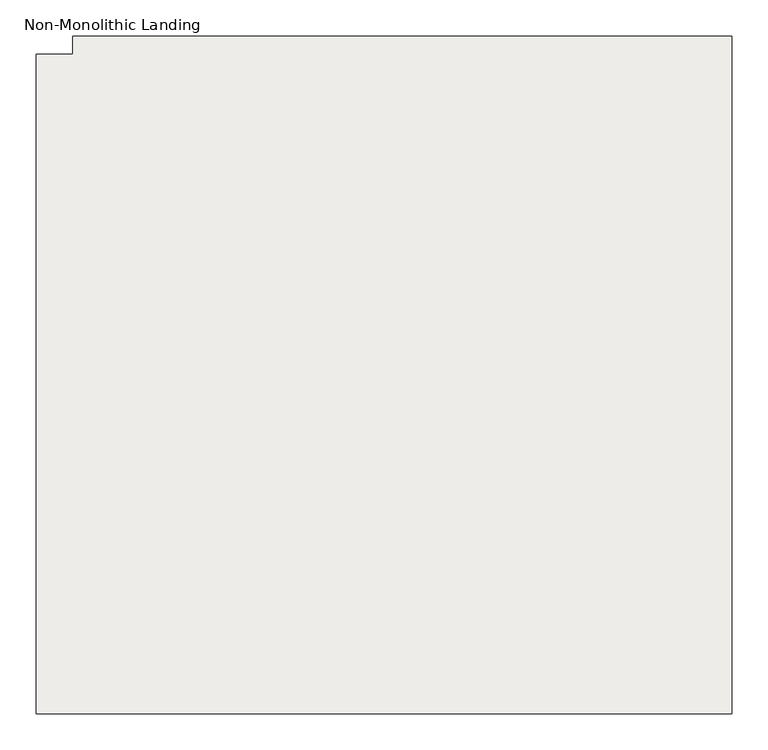
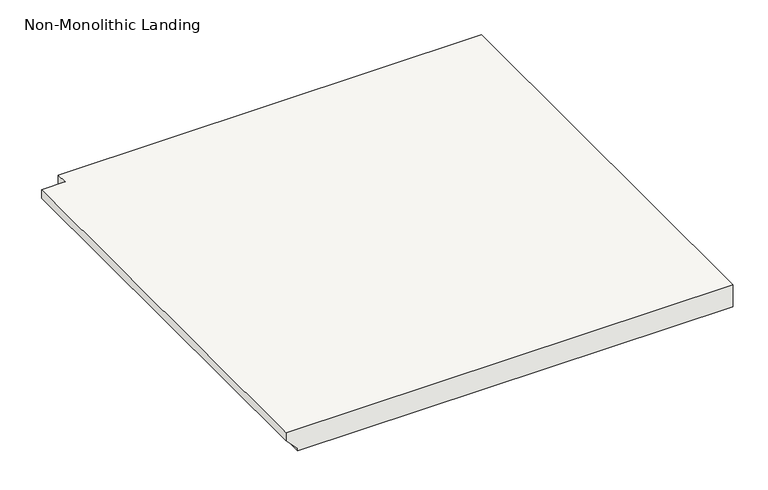
"""IFC4 building model written with IfcOpenShell, lengths in millimetres: slab geometry, Non-Monolithic Landing."""

from ifc_helpers import new_model, si_unit, origin, place, context, project, spatial, faceted_brep, source, transform, mapped, element, save


def non_monolithic_landing_5acc3baf(model_context):
    return source(origin(), model_context, "Body", "Brep", [
        faceted_brep([(-1954.0563134, -12709.459218, 4044.95), (-1954.0563134, -12709.459218, 4064.0), (-1954.0563134, -11795.059218, 4064.0), (-1954.0563134, -11795.059218, 4044.95), (-1928.6563134, -12709.459218, 4019.55), (-1928.6563134, -11795.059218, 4019.55), (-988.8563134, -12709.459218, 4064.0), (-988.8563134, -11795.059218, 4064.0), (-988.8563134, -11769.659218, 4064.0), (-1903.2563134, -11769.659218, 4064.0), (-1903.2563134, -11795.059218, 4064.0), (-1928.6563134, -12709.459218, 4013.2), (-1928.6563134, -11795.059218, 4013.2), (-1903.2563134, -11795.059218, 4013.2), (-1903.2563134, -11769.659218, 4013.2), (-988.8563134, -11769.659218, 4013.2), (-988.8563134, -11795.059218, 4013.2), (-988.8563134, -12709.459218, 4013.2)], [[[0, 1, 2, 3]], [[4, 0, 3, 5]], [[6, 7, 8, 9, 10, 2, 1]], [[11, 12, 13, 14, 15, 16, 17]], [[12, 11, 4, 5]], [[6, 1, 0, 4, 11, 17]], [[7, 6, 17, 16]], [[8, 7, 16, 15]], [[9, 8, 15, 14]], [[10, 9, 14, 13]], [[2, 10, 13, 12, 5, 3]]]),
    ])


if __name__ == "__main__":
    model = new_model("IFC4")
    model_context = context("Model", 3, world=origin())
    ifc_project = project(units=[si_unit("LENGTHUNIT", "METRE", prefix="MILLI")], contexts=[model_context])
    site = spatial("IfcSite", under=ifc_project)
    building = spatial("IfcBuilding", under=site)
    placement = place(None, origin())
    non_monolithic_landing_shape = non_monolithic_landing_5acc3baf(model_context)
    element("IfcSlab", 1, ObjectType="Non-Monolithic Landing", at=placement, inside=building, context=model_context, shape_type="MappedRepresentation", body=[
        mapped(non_monolithic_landing_shape, transform((0.0, 0.0, 0.0), x_axis=(1.0, 0.0, 0.0), y_axis=(0.0, 1.0, 0.0), z_axis=(0.0, 0.0, 1.0))),
    ])
    save(model, "model.ifc")
